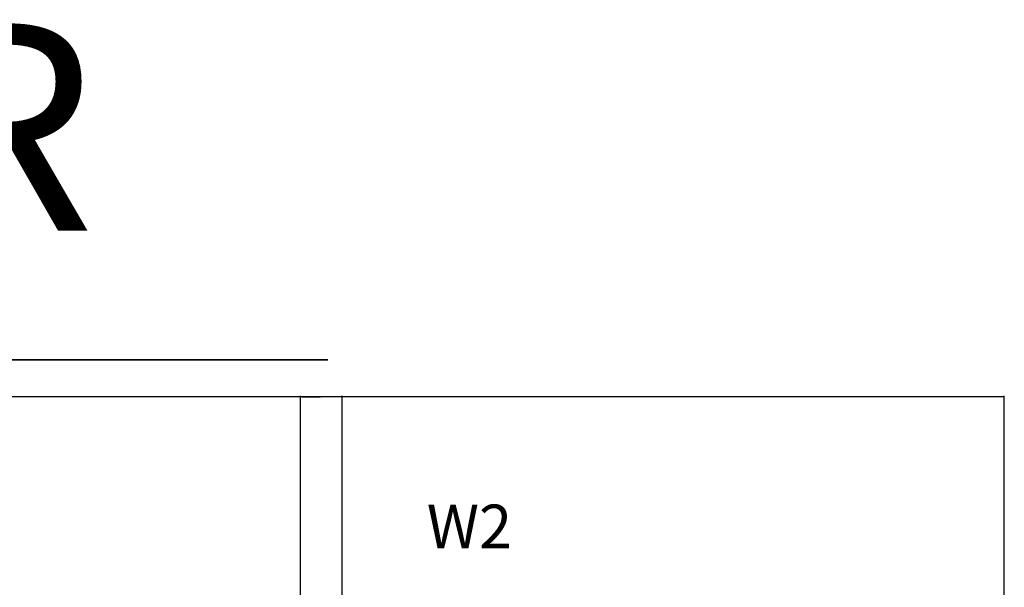
# Model space of a CAD drawing. Units: inches. Extents: x 7359 to 7979, y 33027 to 34263.
# Tile 29 of 32: x 7753 to 7894, y 33630 to 33711. Entities that reach past the tile are written whole.
import ezdxf

# ---------------------------------------------------------------- set-up
doc = ezdxf.new("R2010")
doc.units = ezdxf.units.IN
for name, color, linetype, lineweight in [('A-ANNO-DIMS', 2, 'Continuous', 18), ('A-ANNO-TEXT', 3, 'Continuous', 18), ('A-ANNO-TITL', 7, 'Continuous', 35)]:
    doc.layers.add(name, color=color, linetype=linetype, lineweight=lineweight)
doc.styles.get("Standard").update_dxf_attribs({"font": 'arial.ttf'})
doc.dimstyles.get("Standard").update_dxf_attribs({"dimtxt": 0.18, "dimasz": 0.18, "dimexe": 0.18, "dimexo": 0.0625, "dimgap": 0.09, "dimtad": 0, "dimtih": 1, "dimtoh": 1, "dimdec": 4, "dimzin": 0, "dimdsep": 46, "dimtxsty": 'Standard', "dimcen": 0.09, "dimadec": 0, "dimazin": 0, "dimtfac": 1, "dimtdec": 4, "dimtofl": 0, "dimtmove": 0, "dimatfit": 3, "dimfxl": 1, "dimtolj": 1, "dimtzin": 0, "dimarcsym": 0})

# ---------------------------------------------------------------- blocks, each defined once
blk = doc.blocks.new('*D66')
at = {"layer": 'A-ANNO-DIMS', "color": 0, "lineweight": -2, "transparency": 16777216}
for p, q in [((7468.73, 33627.22), (7468.73, 33657.24)), ((7468.91, 33657.06), (7681.03, 33657.06)), ((7893.95, 33657.06), (7681.82, 33657.06)), ((7894.13, 33627.22), (7894.13, 33657.24))]:
    blk.add_line(p, q, dxfattribs=at)
at = {"layer": 'A-ANNO-DIMS', "color": 0, "transparency": 16777216}
for points in [[(7468.91, 33657.09), (7468.91, 33657.03), (7468.73, 33657.06)], [(7893.95, 33657.09), (7893.95, 33657.03), (7894.13, 33657.06)]]:
    blk.add_solid(points, dxfattribs=at)
at = {"layer": 'Defpoints', "color": 0, "transparency": 16777216}
for p in [(7894.13, 33657.06), (7468.73, 33627.16), (7894.13, 33627.16)]:
    blk.add_point(p, dxfattribs=at)
at = {"layer": 'A-ANNO-DIMS', "color": 0, "transparency": 16777216, "insert": (7681.43, 33657.06), "char_height": 0.18, "attachment_point": 5}
blk.add_mtext('\\A1;425.4', dxfattribs=at)
blk = doc.blocks.new('*D88')
at = {"layer": 'A-ANNO-DIMS', "color": 0, "lineweight": -2, "transparency": 16777216}
for p, q in [((7793.126578, 33448.724789), (7793.126578, 33657.242289)), ((7793.306578, 33657.062289), (7795.977151, 33657.062289)), ((7798.946578, 33657.062289), (7796.276005, 33657.062289)), ((7799.126578, 33448.724789), (7799.126578, 33657.242289))]:
    blk.add_line(p, q, dxfattribs=at)
at = {"layer": 'A-ANNO-DIMS', "color": 0, "transparency": 16777216}
for points in [[(7793.306578, 33657.092289), (7793.306578, 33657.032289), (7793.126578, 33657.062289)], [(7798.946578, 33657.092289), (7798.946578, 33657.032289), (7799.126578, 33657.062289)]]:
    blk.add_solid(points, dxfattribs=at)
at = {"layer": 'Defpoints', "color": 0, "transparency": 16777216}
for p in [(7799.126578, 33657.062289), (7793.126578, 33448.662289), (7799.126578, 33448.662289)]:
    blk.add_point(p, dxfattribs=at)
at = {"layer": 'A-ANNO-DIMS', "color": 0, "transparency": 16777216, "insert": (7796.126578, 33657.062289), "char_height": 0.18, "attachment_point": 5}
blk.add_mtext('\\A1;6', dxfattribs=at)

msp = doc.modelspace()

# ---------------------------------------------------------------- linework, layer by layer
at = {"layer": 'A-ANNO-TITL'}
msp.add_line((7519.7539, 33662.3891), (7797.0359, 33662.3891), dxfattribs=at)

# ---------------------------------------------------------------- texts
at = {"layer": 'A-ANNO-TEXT'}
msp.add_text('W2', height=6.25941, dxfattribs=at).set_placement((7811.2574, 33635.3495))
at = {"layer": 'A-ANNO-TITL'}
msp.add_text('FIRST FLOOR', height=29.769676, dxfattribs=at).set_placement((7515.4376, 33680.9181))

# ---------------------------------------------------------------- dimensions: what is measured, and where the dimension line sits
at = {"layer": 'A-ANNO-DIMS'}
for base, p1, p2, override, picture, middle in [((7894.1266, 33657.0623), (7468.7266, 33627.1623), (7894.1266, 33627.1623), {"dimdec": 1, "dimlfac": 1, "dimrnd": 0, "dimzin": 0, "dimdsep": 46, "dimlunit": 2}, '*D66', (7681.4266, 33657.0623)), ((7799.1266, 33657.0623), (7793.1266, 33448.6623), (7799.1266, 33448.6623), {"dimdec": 0, "dimlfac": 1, "dimrnd": 0, "dimzin": 0, "dimdsep": 46, "dimlunit": 2}, '*D88', (7796.1266, 33657.0623))]:
    dim = msp.add_linear_dim(base=base, p1=p1, p2=p2, dimstyle='Standard', override=override, dxfattribs=at)
    dim.commit()
    dim.dimension.update_dxf_attribs({"geometry": picture, "text_midpoint": middle})

doc.saveas('drawing.dxf')
